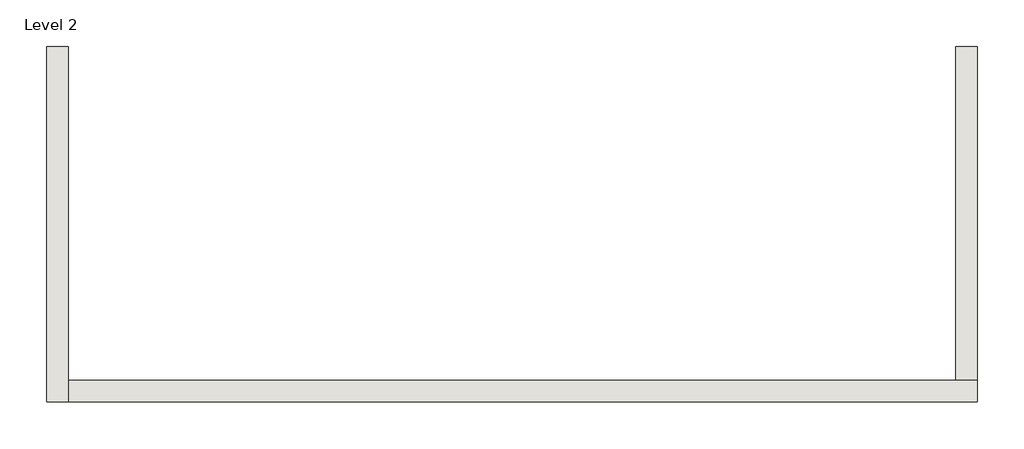
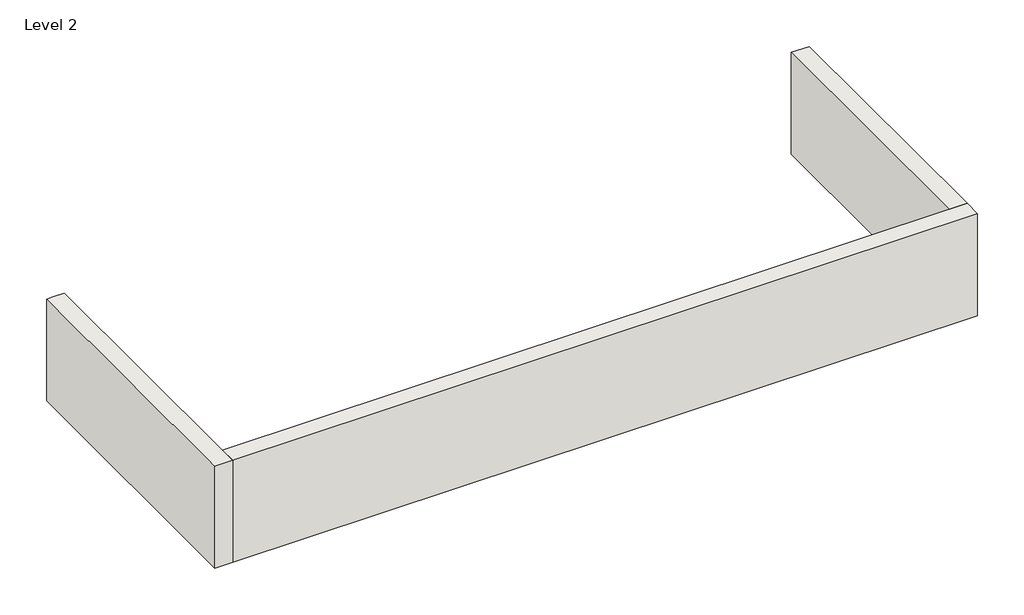
# One storey: 3 walls.
"""IFC4 building model written with IfcOpenShell, lengths in millimetres."""

from ifc_helpers import new_model, si_unit, frame, origin, place, context, project, spatial, polyline, outline, extrude, faceted_brep, element, save

model = new_model("IFC4")

# Units and contexts
model_context = context("Model", 3, world=origin())
ifc_project = project(units=[si_unit("LENGTHUNIT", "METRE", prefix="MILLI")], contexts=[model_context])

# Site, building, storey
site = spatial("IfcSite", under=ifc_project)
building = spatial("IfcBuilding", under=site)
storey = spatial("IfcBuildingStorey", under=building, Name="Level 2", Elevation=3657.6)

# Walls
placement = place(None, origin())
element("IfcWall", 1, ObjectType="4.5\" wall", at=placement, inside=storey, context=model_context, shape_type="Brep", body=[
    faceted_brep([(-12197.4679297, -85.3803708, 3048.0), (-12197.4679297, -1736.3803708, 3048.0), (-12197.4679297, -1736.3803708, 3657.6), (-12197.4679297, -85.3803708, 3657.6), (-12095.8679297, -85.3803708, 3048.0), (-12095.8679297, -85.3803708, 3657.6), (-12095.8679297, -1634.7803708, 3657.6), (-12095.8679297, -1736.3803708, 3657.6), (-12095.8679297, -1736.3803708, 3048.0), (-12095.8679297, -1634.7803708, 3048.0), (-12159.3679297, -85.3803708, 3657.6)], [[[0, 1, 2, 3]], [[4, 5, 6, 7, 8, 9]], [[1, 0, 4, 9, 8]], [[3, 2, 7, 6, 5, 10]], [[2, 1, 8, 7]], [[0, 3, 10, 5, 4]]]),
])
element("IfcWall", 2, ObjectType="4.5\" wall", at=placement, inside=storey, context=model_context, shape_type="Brep", body=[
    faceted_brep([(-12095.8679297, -1736.3803708, 3048.0), (-7879.4679297, -1736.3803708, 3048.0), (-7879.4679297, -1736.3803708, 3657.6), (-12095.8679297, -1736.3803708, 3657.6), (-12095.8679297, -1634.7803708, 3048.0), (-12095.8679297, -1634.7803708, 3657.6), (-7981.0679297, -1634.7803708, 3657.6), (-7879.4679297, -1634.7803708, 3657.6), (-7879.4679297, -1634.7803708, 3048.0), (-7981.0679297, -1634.7803708, 3048.0)], [[[0, 1, 2, 3]], [[4, 5, 6, 7, 8, 9]], [[1, 0, 4, 9, 8]], [[3, 2, 7, 6, 5]], [[0, 3, 5, 4]], [[2, 1, 8, 7]]]),
])
element("IfcWall", 3, ObjectType="4.5\" wall", at=placement, inside=storey, context=model_context, shape_type="SweptSolid", body=[
    extrude(outline(polyline([(-7879.4679297, -85.3803708), (-7879.4679297, -1634.7803708), (-7981.0679297, -1634.7803708), (-7981.0679297, -85.3803708), (-7879.4679297, -85.3803708)])), frame((0.0, 0.0, 3048.0), z_axis=(0.0, 0.0, 1.0), x_axis=(1.0, 0.0, 0.0)), (0.0, 0.0, 1.0), 609.6),
])

save(model, "model.ifc")

# Revit data of these elements
# Type "4.5\" wall"
#   Assembly Code = "B2010"
#   Layers, outside or top first: 0' - 4" "Laminate, Ivory, Matte" (function 1)
# Elements 1, 2, 3 (IfcWall, "4.5\" wall")
#   built-in parameter 1001111 = -2' - 0"
#   Top Offset = -0' - 6"
#   Base Offset = -2' - 0"
#   wall height = 2' - 0"
#   Phase Created = New Construction
#   Base Constraint = Level 2
#   Top Constraint = Level 3
#   Materials on its faces: "Laminate, Ivory, Matte"
# Materials
#   "Laminate, Ivory, Matte": class "Plastic", colour RGB 247 247 239, transparency 0, Description = "Plastic Laminate - Ivory, Matte", Cost = 0
